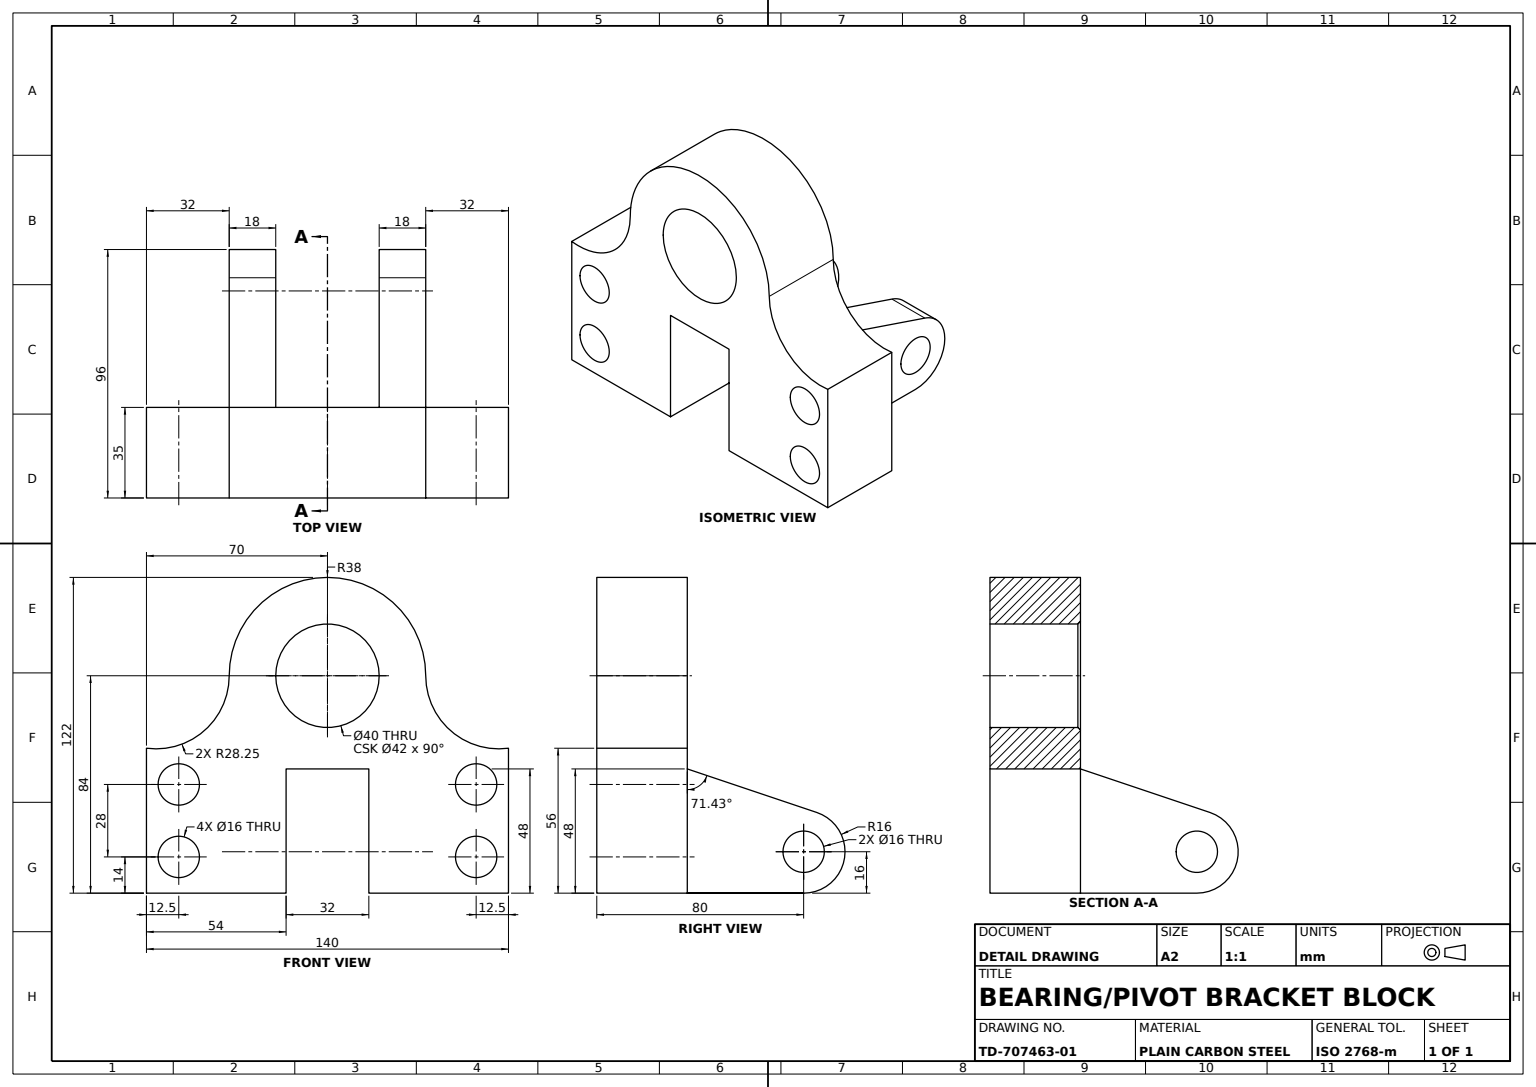
SolidWorks part; units mm, degrees
material "Plain Carbon Steel"
ref_plane "Front Plane" through (0, 0, 0) normal (0, 0, 1) x (1, 0, 0)
ref_plane "Top Plane" through (0, 0, 0) normal (0, 1, 0) x (1, 0, 0)
ref_plane "Right Plane" through (0, 0, 0) normal (1, 0, 0) x (0, 0, -1)
sketch "Base Block Profile" plane through (0, 0, 0) normal (0, 0, 1) x (1, 0, 0)
  line L0 (-70, -28) -> (-70, -84)
  line L1 (-70, -84) -> (70, -84)
  line L2 (70, -84) -> (70, -28)
  arc A0 (38, 0) -> (-38, 0) centre (0, 0) ccw
  arc A2 (-70, -28) -> (-38, 0) centre (-66.25, 0) ccw
  arc A3 (38, 0) -> (70, -28) centre (66.25, 0) ccw
  dimension "D1" = 38
  dimension "D2" = 56
  dimension "D3" = 70
  dimension "D4" = 70
  dimension "D5" = 28.25
  dimension "D6" = 28.25
  dimension "D7" = 56
extrude "Base Block" add sketch "Base Block Profile" along normal blind 35
sketch "Bore Profile" plane through (0, 0, 35) normal (0, 0, 1) x (1, 0, 0)
  circle A0 centre (0, 0) radius 20
  dimension "D1" = 40
extrude "Bore Ø40" cut sketch "Bore Profile" against normal blind 35
sketch "Mounting Holes Profile" plane through (0, 0, 35) normal (0, 0, 1) x (1, 0, 0)
  line L0 (-70, -28) -> (-70, -84) construction
  line L1 (70, -84) -> (70, -28) construction
  circle A0 centre (-57.5, -42) radius 8
  circle A1 centre (-57.5, -70) radius 8
  circle A2 centre (57.5, -42) radius 8
  circle A3 centre (57.5, -70) radius 8
  dimension "D1" = 16
  dimension "D2" = 16
  dimension "D3" = 16
  dimension "D4" = 16
  dimension "D8" = 12.5
  dimension "D9" = 28
  dimension "D10" = 12.5
  dimension "D11" = 14
  dimension "D12" = 28
  dimension "D5" = 12.5
  dimension "D6" = 12.5
  dimension "D7" = 14
extrude "Mounting Holes 4x" cut sketch "Mounting Holes Profile" against normal blind 35
ref_plane "Side Arm Plane" through (38, 0, 0) normal (1, 0, 0) x (0, 0, -1)
sketch "Side Arm Profile" plane through (38, 0, 0) normal (1, 0, 0) x (0, 0, -1)
  line L0 (0, -84) -> (0, -36)
  line L1 (0, -28.25) -> (0, 0) construction
  line L2 (0, -36) -> (50.0963, -52.8333)
  line L3 (0, -84) -> (45, -84)
  line L4 (-35, -84) -> (-35, -28) construction
  arc A2 (45, -84) -> (50.0963, -52.8333) centre (45, -68) ccw
  circle A3 centre (45, -68) radius 8
  dimension "D3" = 16
  dimension "D4" = 80
  dimension "D2" = 16
  dimension "D1" = 48
extrude "Side Arm" add sketch "Side Arm Profile" against normal blind 18
ref_plane "Lug Plane" through (-38, 0, 0) normal (1, 0, 0) x (0, 0, -1)
sketch "Lug Boss Profile" plane through (-38, 0, 0) normal (1, 0, 0) x (0, 0, -1)
  line L0 (0, -36) -> (0, -84) construction
  line L1 (0, -84) -> (45, -84) construction
  line L2 (50.0963, -52.8333) -> (0, -36) construction
  line L3 (0, -36) -> (0, -84)
  line L4 (0, -84) -> (45, -84)
  line L5 (50.0963, -52.8333) -> (0, -36)
  circle A0 centre (45, -68) radius 8 construction
  arc A1 (45, -84) -> (50.0963, -52.8333) centre (45, -68) ccw construction
  circle A2 centre (45, -68) radius 8
  arc A3 (45, -84) -> (50.0963, -52.8333) centre (45, -68) ccw
extrude "Lug Boss" add sketch "Lug Boss Profile" along normal blind 18
sketch "Relief Cut Profile" plane through (0, 0, 0) normal (0, 0, -1) x (-1, 0, 0)
  line L0 (-16, -84) -> (16, -84)
  line L1 (20, -84) -> (-20, -84) construction
  line L2 (16, -84) -> (16, -36)
  line L5 (16, -36) -> (-16, -36)
  line L6 (-16, -36) -> (-16, -84)
  line L7 (20, -52.8333) -> (20, -84) construction
  dimension "D1" = 32
  dimension "D2" = 4
  dimension "D3" = 48
extrude "Relief Cut" cut sketch "Relief Cut Profile" against normal blind 35
chamfer "Bore Chamfer 1mm" distance 1 angle 45 1 edges at (20, 0, 0)
